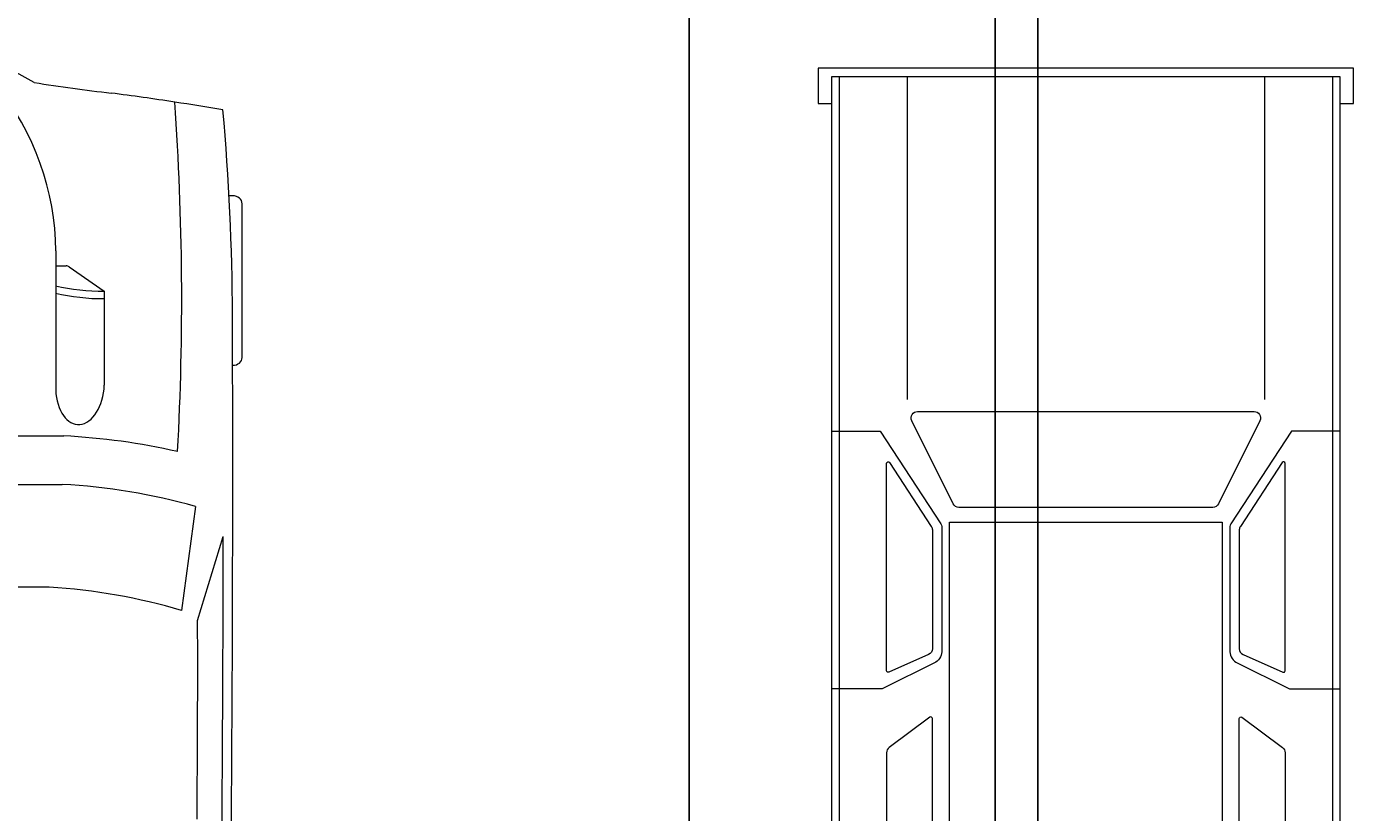
# Model space of a CAD drawing. Units: inches. Extents: x 5375 to 6084, y 16106 to 17259.
# Tile 11 of 32: x 5844 to 5984, y 16295 to 16377. Entities that reach past the tile are written whole.
import ezdxf

# ---------------------------------------------------------------- set-up
doc = ezdxf.new("R2010")
doc.units = ezdxf.units.IN
doc.layers.add('A-ANNO-DIMS', color=2, linetype='Continuous', lineweight=18)
doc.layers.add('C-PKNG-VEHI', color=7, linetype='Continuous', lineweight=13)
doc.styles.get("Standard").update_dxf_attribs({"font": 'arial.ttf'})
doc.dimstyles.get("Standard").update_dxf_attribs({"dimtxt": 0.18, "dimasz": 0.18, "dimexe": 0.18, "dimexo": 0.0625, "dimgap": 0.09, "dimtad": 0, "dimtih": 1, "dimtoh": 1, "dimdec": 4, "dimzin": 0, "dimdsep": 46, "dimtxsty": 'Standard', "dimcen": 0.09, "dimadec": 0, "dimazin": 0, "dimtfac": 1, "dimtdec": 4, "dimtofl": 0, "dimtmove": 0, "dimatfit": 3, "dimfxl": 1, "dimtolj": 1, "dimtzin": 0, "dimarcsym": 0})

# ---------------------------------------------------------------- blocks, each defined once
blk = doc.blocks.new('*U9')
for p, q in [((46.55, 38.89), (22.35, 38.89)), ((21.1, 37.41), (21.1, 36.83)), ((47.8, 37.39), (47.8, 37.41)), ((87.99, 31.87), (74.76, 35.92)), ((70.03, 31.54), (86.41, 29.35)), ((32.27, 11.63), (36.13, 17.17)), ((36.13, 17.17), (50.94, 17.17)), ((32.12, 9.51), (32.12, 11.15)), ((58.92, -10.77), (58.92, 10.77)), ((66.55, -10.53), (66.55, 10.53)), ((29.77, 9.51), (51.68, 9.51)), ((82.74, 8.5), (82.74, -8.5)), ((3.27, 6.13), (0.1, 0.41))]:
    blk.add_line(p, q)
for centre, major_axis, ratio, start_param, end_param in [((22.35, 37.41), (0, -1.48), 0.842304, 3.141593, 4.712389), ((46.55, 37.41), (0, 1.48), 0.842304, -1.570796, 0), ((266.03, -27.52), (0, 313.31), 0.842304, 1.367076, 1.39176), ((41.19, -490.86), (0, 528.23), 0.842304, 0.00281, 0.075598), ((64.48, -10555.62), (0, 10593.03), 0.842304, -0.013397, 0.002797), ((64.48, -10555.62), (0, -10591.55), 0.842304, 3.133765, 3.140441), ((135.29, 5.39), (0, 81.77), 0.842304, 1.245306, 1.50788), ((95.79, -3666.35), (0, -3698.24), 0.842304, 3.134049, 3.144098), ((37.47, -593.96), (0, -623.33), 0.842304, 3.096046, 3.200911), ((149.6, 2.8), (0, -79.58), 0.842304, 4.372215, 4.640744), ((259.18, -27.52), (0, -305.3), 0.842304, 4.528606, 4.561838), ((134.4, 5.39), (0, -89.78), 0.842304, 4.449482, 4.652344), ((-204.49, 52.4), (0, -250.96), 0.842304, 1.385369, 1.434372), ((13.04, 17.01), (0, 27.42), 0.842304, 4.435146, 4.718221), ((14.2, 17.01), (0, 27.42), 0.842304, 4.435146, 4.718221), ((50.79, 13.34), (6.34, -0.36), 0.603834, -1.395552, 1.581315), ((32.75, 11.15), (0, 0.74), 0.842304, 0.879714, 1.570796), ((29.77, -46.66), (0, 56.17), 0.842304, 0, 0.590319)]:
    blk.add_ellipse(centre, major_axis=major_axis, ratio=ratio, start_param=start_param, end_param=end_param)
blk = doc.blocks.new('*U10')
for p, q in [((1.28, 38.87), (175.66, 38.87)), ((1.28, 28.15), (52.13, 28.15)), ((1.28, -28.15), (52.13, -28.15)), ((1.28, -38.87), (175.66, -38.87))]:
    blk.add_line(p, q)
for points in [[(5.57, 40.01), (5.57, 42.18), (0, 42.18), (0, -42.18), (5.57, -42.18), (5.57, -40.01), (1.28, -40.01), (1.28, 40.01)], [(1.28, 40.01), (175.66, 40.01), (175.66, -40.01), (1.28, -40.01)], [(71.47, 21.48), (163.42, 21.48), (163.42, -21.48), (71.47, -21.48)]]:
    blk.add_lwpolyline(points, close=True)
for points in [[(57.15, 40.01), (57.15, 32.39), (71.72, 22.83, 0.086577), (72.56, 22.68), (91.59, 22.68, 0.227875), (93.54, 23.62), (97.72, 32.11), (97.72, 40.01)], [(57.15, -40.01), (57.15, -32.39), (71.72, -22.83, -0.086577), (72.56, -22.68), (91.59, -22.68, -0.227875), (93.54, -23.62), (97.72, -32.11), (97.72, -40.01)]]:
    blk.add_lwpolyline(points, format="xyb")
for points in [[(62.08, 30.95), (72.14, 24.35, 0.146139), (72.69, 24.18), (91.42, 24.18, 0.29766), (92.33, 24.78), (95.09, 31.05, 0.541236), (94.86, 31.41), (62.21, 31.41, 0.744989)], [(102.19, 24.58), (106.97, 31, -0.236929), (107.78, 31.41), (162.91, 31.41, -0.621576), (163.11, 31), (158.19, 24.58, -0.233368), (157.39, 24.18), (102.39, 24.18, -0.616908)], [(55.49, 27.42), (68.59, 20.89, -0.284287), (69.14, 19.99), (69.14, -19.99, -0.284287), (68.59, -20.89), (55.49, -27.42, -0.557284), (54.05, -26.53), (54.05, 26.53, -0.557284)], [(62.08, -30.95), (72.14, -24.35, -0.146139), (72.69, -24.18), (91.42, -24.18, -0.29766), (92.33, -24.78), (95.09, -31.05, -0.541236), (94.86, -31.41), (62.21, -31.41, -0.744989)], [(102.19, -24.58), (106.97, -31, 0.236929), (107.78, -31.41), (162.91, -31.41, 0.621576), (163.11, -31), (158.19, -24.58, 0.233368), (157.39, -24.18), (102.39, -24.18, 0.616908)]]:
    blk.add_lwpolyline(points, format="xyb", close=True)
blk = doc.blocks.new('*D44')
at = {"layer": 'A-ANNO-DIMS', "color": 0, "lineweight": -2, "transparency": 16777216}
for p, q in [((5914, 16886.53), (5914, 16106.48)), ((5946.12, 16886.53), (5946.12, 16106.48)), ((5914.18, 16106.66), (5929.6, 16106.66)), ((5945.94, 16106.66), (5930.53, 16106.66))]:
    blk.add_line(p, q, dxfattribs=at)
at = {"layer": 'A-ANNO-DIMS', "color": 0, "transparency": 16777216}
for points in [[(5914.18, 16106.69), (5914.18, 16106.63), (5914, 16106.66)], [(5945.94, 16106.69), (5945.94, 16106.63), (5946.12, 16106.66)]]:
    blk.add_solid(points, dxfattribs=at)
at = {"layer": 'Defpoints', "color": 0, "transparency": 16777216}
for p in [(5914, 16886.6), (5946.12, 16886.6), (5914, 16106.66)]:
    blk.add_point(p, dxfattribs=at)
at = {"layer": 'A-ANNO-DIMS', "color": 0, "transparency": 16777216, "insert": (5930.06, 16106.66), "char_height": 0.18, "attachment_point": 5}
blk.add_mtext('\\A1;32.117', dxfattribs=at)
blk = doc.blocks.new('*D46')
at = {"layer": 'A-ANNO-DIMS', "color": 0, "lineweight": -2, "transparency": 16777216}
for p, q in [((5946.12, 16771.52), (5946.12, 16106.48)), ((5950.62, 16771.52), (5950.62, 16106.48)), ((5946.3, 16106.66), (5948.11, 16106.66)), ((5950.44, 16106.66), (5948.63, 16106.66))]:
    blk.add_line(p, q, dxfattribs=at)
at = {"layer": 'A-ANNO-DIMS', "color": 0, "transparency": 16777216}
for points in [[(5946.3, 16106.69), (5946.3, 16106.63), (5946.12, 16106.66)], [(5950.44, 16106.69), (5950.44, 16106.63), (5950.62, 16106.66)]]:
    blk.add_solid(points, dxfattribs=at)
at = {"layer": 'Defpoints', "color": 0, "transparency": 16777216}
for p in [(5946.12, 16771.58), (5950.62, 16771.58), (5950.62, 16106.66)]:
    blk.add_point(p, dxfattribs=at)
at = {"layer": 'A-ANNO-DIMS', "color": 0, "transparency": 16777216, "insert": (5948.37, 16106.66), "char_height": 0.18, "attachment_point": 5}
blk.add_mtext('\\A1;4.5', dxfattribs=at)

msp = doc.modelspace()

# ---------------------------------------------------------------- block references
at = {"layer": 'C-PKNG-VEHI', "xscale": 0.6659567702331713, "yscale": 0.6659567702331713, "zscale": 0.6659567702331713, "rotation": 270}
for name, p in [('*U9', (5841.1969, 16373.5119)), ('*U10', (5955.6438, 16372.8314))]:
    msp.add_blockref(name, p, dxfattribs=at)

# ---------------------------------------------------------------- dimensions: what is measured, and where the dimension line sits
at = {"layer": 'A-ANNO-DIMS'}
for base, p1, p2, override, picture, middle in [((5914.0033, 16106.6631), (5946.1199, 16886.5956), (5914.0033, 16886.5956), {"dimdec": 3, "dimlfac": 1, "dimrnd": 0, "dimzin": 0, "dimdsep": 46, "dimlunit": 2}, '*D44', (5930.0616, 16106.6631)), ((5950.6199, 16106.6631), (5946.1199, 16771.5793), (5950.6199, 16771.5793), {"dimdec": 1, "dimlfac": 1, "dimrnd": 0, "dimzin": 0, "dimdsep": 46, "dimlunit": 2}, '*D46', (5948.3699, 16106.6631))]:
    dim = msp.add_linear_dim(base=base, p1=p1, p2=p2, dimstyle='Standard', override=override, dxfattribs=at)
    dim.commit()
    dim.dimension.update_dxf_attribs({"geometry": picture, "text_midpoint": middle})

doc.saveas('drawing.dxf')
